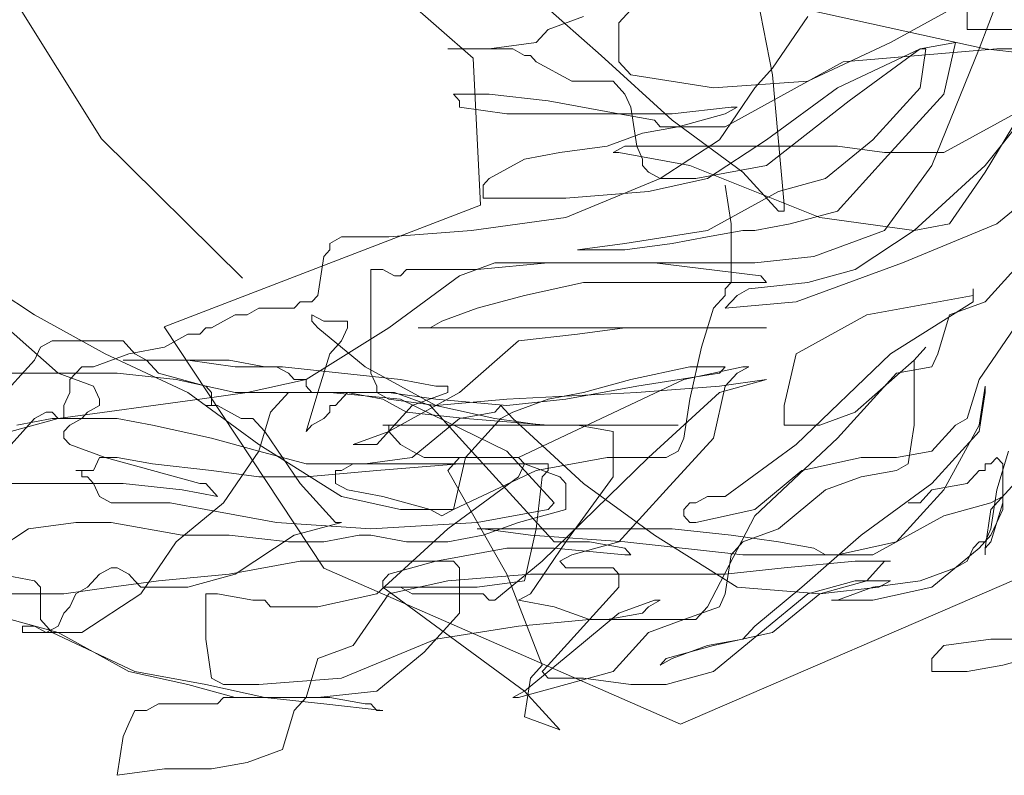
# Model space of a CAD drawing. Units: inches. Extents: x 1994 to 3075, y 3517 to 3950.
# Tile 38 of 58: x 1994.64257 to 1994.647842, y 3553.737841 to 3553.741889. Entities that reach past the tile are written whole.
import ezdxf

# ---------------------------------------------------------------- set-up
doc = ezdxf.new("R2010")
doc.units = ezdxf.units.IN
doc.layers.add('A-FURN-REFR', color=8, linetype='Continuous', lineweight=13)

msp = doc.modelspace()

# ---------------------------------------------------------------- linework, layer by layer
at = {"layer": 'A-FURN-REFR'}
for p, q in [((1994.6419152, 3553.7430024), (1994.6430076, 3553.7412502)), ((1994.6449987, 3553.7416831), (1994.6436467, 3553.7428672)), ((1994.6466007, 3553.741594), (1994.6464111, 3553.7425669)), ((1994.6480232, 3553.7425669), (1994.647707, 3553.741733)), ((1994.6476438, 3553.742289), (1994.6476438, 3553.7418372)), ((1994.6453679, 3553.7419762), (1994.645684, 3553.7416983)), ((1994.6476122, 3553.7419762), (1994.6472329, 3553.7417677)), ((1994.6453996, 3553.7418372), (1994.6455892, 3553.7419067)), ((1994.6457789, 3553.741872), (1994.6458421, 3553.7419415)), ((1994.6467904, 3553.7419067), (1994.6466007, 3553.7416288)), ((1994.6467904, 3553.7419415), (1994.6477386, 3553.741733)), ((1994.6453363, 3553.7417677), (1994.6453996, 3553.7418372)), ((1994.6457789, 3553.7416635), (1994.6457789, 3553.741872)), ((1994.6476438, 3553.7418372), (1994.6480548, 3553.7418372)), ((1994.6448622, 3553.741733), (1994.6450834, 3553.741733)), ((1994.6452099, 3553.741733), (1994.6448622, 3553.741733)), ((1994.6450834, 3553.741733), (1994.6453363, 3553.7417677)), ((1994.6452731, 3553.7416983), (1994.6452099, 3553.741733)), ((1994.6472329, 3553.7417677), (1994.6467904, 3553.7415593)), ((1994.6469484, 3553.7415245), (1994.647391, 3553.741733)), ((1994.6478019, 3553.741733), (1994.64698, 3553.7416635)), ((1994.647391, 3553.741733), (1994.6470116, 3553.741455)), ((1994.647391, 3553.741733), (1994.6475806, 3553.7417677)), ((1994.6474226, 3553.741733), (1994.647391, 3553.741733)), ((1994.647391, 3553.7415245), (1994.6474226, 3553.741733)), ((1994.647707, 3553.741733), (1994.6474542, 3553.7411075)), ((1994.6475806, 3553.7417677), (1994.6475174, 3553.7414898)), ((1994.6477386, 3553.741733), (1994.6483708, 3553.7416635)), ((1994.6483708, 3553.741733), (1994.6478019, 3553.741733)), ((1994.6450375, 3553.7408956), (1994.6449987, 3553.7416831)), ((1994.6453047, 3553.7416983), (1994.6452731, 3553.7416983)), ((1994.6453363, 3553.7416635), (1994.6453047, 3553.7416983)), ((1994.645684, 3553.7416983), (1994.6460633, 3553.7413508)), ((1994.645526, 3553.7415593), (1994.6453363, 3553.7416635)), ((1994.6458421, 3553.741594), (1994.6457789, 3553.7416635)), ((1994.64698, 3553.7416635), (1994.6463478, 3553.741316)), ((1994.6466007, 3553.7416288), (1994.6465059, 3553.7415245)), ((1994.6481812, 3553.7416635), (1994.6477386, 3553.7411075)), ((1994.6462846, 3553.7415245), (1994.6458421, 3553.741594)), ((1994.6466639, 3553.7408991), (1994.6466007, 3553.741594)), ((1994.6457472, 3553.7415593), (1994.645526, 3553.7415593)), ((1994.6458105, 3553.7414898), (1994.6457472, 3553.7415593)), ((1994.6467904, 3553.7415593), (1994.6462846, 3553.7415245)), ((1994.6465059, 3553.7415245), (1994.6463162, 3553.7412465)), ((1994.6465691, 3553.7412465), (1994.6469484, 3553.7415245)), ((1994.6471381, 3553.7412465), (1994.647391, 3553.7415245)), ((1994.6448938, 3553.7414898), (1994.6449254, 3553.741455)), ((1994.6450834, 3553.7414898), (1994.6448938, 3553.7414898)), ((1994.6453996, 3553.741455), (1994.6450834, 3553.7414898)), ((1994.6458421, 3553.7414202), (1994.6458105, 3553.7414898)), ((1994.6475174, 3553.7414898), (1994.6472013, 3553.7411423)), ((1994.6477386, 3553.7410728), (1994.6479915, 3553.7414898)), ((1994.6449254, 3553.741455), (1994.6449254, 3553.7414202)), ((1994.6449254, 3553.7414202), (1994.6451783, 3553.7413855)), ((1994.6457789, 3553.7413855), (1994.6453996, 3553.741455)), ((1994.6458737, 3553.7412118), (1994.6458421, 3553.7414202)), ((1994.6460633, 3553.7413855), (1994.6463794, 3553.7414202)), ((1994.6464111, 3553.7414202), (1994.6463478, 3553.7413855)), ((1994.6463794, 3553.7414202), (1994.6464111, 3553.7414202)), ((1994.6470116, 3553.741455), (1994.6465691, 3553.7411075)), ((1994.6480232, 3553.741455), (1994.6475174, 3553.741177)), ((1994.6451783, 3553.7413855), (1994.6460633, 3553.7413855)), ((1994.6459685, 3553.7413508), (1994.6457789, 3553.7413855)), ((1994.6463478, 3553.7413855), (1994.6460949, 3553.741316)), ((1994.6460949, 3553.741316), (1994.6459053, 3553.7412813)), ((1994.6460001, 3553.741316), (1994.6459685, 3553.7413508)), ((1994.6463478, 3553.741316), (1994.6460001, 3553.741316)), ((1994.6460633, 3553.7413508), (1994.6464427, 3553.7410728)), ((1994.6459053, 3553.7412813), (1994.6457156, 3553.7412118)), ((1994.6430076, 3553.7412502), (1994.643763, 3553.7405048)), ((1994.6457156, 3553.7412118), (1994.6454628, 3553.741177)), ((1994.6458105, 3553.7412118), (1994.6457472, 3553.741177)), ((1994.6469484, 3553.7412118), (1994.6458105, 3553.7412118)), ((1994.6459053, 3553.7411423), (1994.6458737, 3553.7412118)), ((1994.6463162, 3553.7412465), (1994.6460001, 3553.741038)), ((1994.646253, 3553.741038), (1994.6465691, 3553.7412465)), ((1994.6468852, 3553.741038), (1994.6471381, 3553.7412465)), ((1994.6472013, 3553.741177), (1994.6469484, 3553.7412118)), ((1994.6454628, 3553.741177), (1994.6452731, 3553.7411423)), ((1994.6457472, 3553.741177), (1994.6457789, 3553.741177)), ((1994.6457789, 3553.741177), (1994.6461582, 3553.7411075)), ((1994.6475174, 3553.741177), (1994.6472013, 3553.741177)), ((1994.6452731, 3553.7411423), (1994.6450834, 3553.741038)), ((1994.6459053, 3553.7411075), (1994.6459053, 3553.7411423)), ((1994.6459369, 3553.7410728), (1994.6459053, 3553.7411075)), ((1994.6461582, 3553.7411075), (1994.6468536, 3553.7408296)), ((1994.6465691, 3553.7411075), (1994.6461898, 3553.741038)), ((1994.6472013, 3553.7411423), (1994.6469484, 3553.7408643)), ((1994.6474542, 3553.7411075), (1994.6472013, 3553.7407601)), ((1994.6477386, 3553.7411075), (1994.6473593, 3553.7407601)), ((1994.6460001, 3553.741038), (1994.6459369, 3553.7410728)), ((1994.6464427, 3553.7410728), (1994.6466323, 3553.7408643)), ((1994.647549, 3553.7407948), (1994.6477386, 3553.7410728)), ((1994.6450834, 3553.741038), (1994.6450518, 3553.7410033)), ((1994.6450518, 3553.7410033), (1994.6450518, 3553.7409338)), ((1994.6460001, 3553.741038), (1994.6454944, 3553.7408296)), ((1994.6459369, 3553.7409686), (1994.646253, 3553.741038)), ((1994.6461898, 3553.741038), (1994.6460001, 3553.741038)), ((1994.6463794, 3553.7407948), (1994.6463478, 3553.7410033)), ((1994.6466323, 3553.7409686), (1994.6468852, 3553.741038)), ((1994.6478019, 3553.7407948), (1994.6480548, 3553.7410033)), ((1994.6454944, 3553.7409338), (1994.6459369, 3553.7409686)), ((1994.646253, 3553.7407601), (1994.6466323, 3553.7409686)), ((1994.6433447, 3553.7402433), (1994.6450375, 3553.7408956)), ((1994.6450518, 3553.7409338), (1994.6454944, 3553.7409338)), ((1994.6466639, 3553.7408643), (1994.6466639, 3553.7408991)), ((1994.6466323, 3553.7408643), (1994.6466639, 3553.7408643)), ((1994.6469484, 3553.7408643), (1994.6466955, 3553.7407948)), ((1994.6454944, 3553.7408296), (1994.6449886, 3553.7407601)), ((1994.6463794, 3553.7404821), (1994.6463794, 3553.7407948)), ((1994.6466955, 3553.7407948), (1994.6465059, 3553.7407601)), ((1994.6468536, 3553.7408296), (1994.6473593, 3553.7407601)), ((1994.6472961, 3553.7405864), (1994.6478019, 3553.7407948)), ((1994.6473593, 3553.7407601), (1994.647549, 3553.7407948)), ((1994.6449886, 3553.7407601), (1994.6445461, 3553.7407253)), ((1994.6458105, 3553.7406905), (1994.646253, 3553.7407601)), ((1994.6464427, 3553.7407601), (1994.646253, 3553.7407253)), ((1994.6465059, 3553.7407601), (1994.6464427, 3553.7407601)), ((1994.6472013, 3553.7407601), (1994.6470116, 3553.7406905)), ((1994.6473593, 3553.7407601), (1994.6470433, 3553.7405516)), ((1994.6442932, 3553.7407253), (1994.64423, 3553.7406905)), ((1994.64423, 3553.7406905), (1994.64423, 3553.7406558)), ((1994.6445461, 3553.7407253), (1994.6442932, 3553.7407253)), ((1994.6455576, 3553.7406558), (1994.6458105, 3553.7406905)), ((1994.6460633, 3553.7406905), (1994.6458105, 3553.7406558)), ((1994.646253, 3553.7407253), (1994.6460633, 3553.7406905)), ((1994.6470116, 3553.7406905), (1994.646822, 3553.7406211)), ((1994.64423, 3553.7406558), (1994.6441984, 3553.7406211)), ((1994.6458105, 3553.7406558), (1994.6455576, 3553.7406558)), ((1994.6441984, 3553.7406211), (1994.6441668, 3553.7404126)), ((1994.645115, 3553.7405864), (1994.6449254, 3553.7405168)), ((1994.6453996, 3553.7405864), (1994.6450202, 3553.7405516)), ((1994.6465059, 3553.7405864), (1994.645115, 3553.7405864)), ((1994.6459685, 3553.7405864), (1994.6453996, 3553.7405864)), ((1994.6465375, 3553.7405168), (1994.6459685, 3553.7405864)), ((1994.646822, 3553.7406211), (1994.6465059, 3553.7405864)), ((1994.6467271, 3553.7403778), (1994.6472961, 3553.7405864)), ((1994.6477386, 3553.7403778), (1994.6479283, 3553.7405864)), ((1994.6444512, 3553.7405516), (1994.6444512, 3553.7399956)), ((1994.6445145, 3553.7405516), (1994.6444512, 3553.7405516)), ((1994.6445777, 3553.7405168), (1994.6445145, 3553.7405516)), ((1994.6446409, 3553.7405516), (1994.6446093, 3553.7405168)), ((1994.6450202, 3553.7405516), (1994.6446409, 3553.7405516)), ((1994.6470433, 3553.7405516), (1994.6467904, 3553.7404821)), ((1994.6423334, 3553.7405168), (1994.6426495, 3553.7403083)), ((1994.6449254, 3553.7405168), (1994.6445461, 3553.7402389)), ((1994.6446093, 3553.7405168), (1994.6445777, 3553.7405168)), ((1994.6452731, 3553.7404126), (1994.6455892, 3553.7404821)), ((1994.6455892, 3553.7404821), (1994.6465691, 3553.7404821)), ((1994.6463478, 3553.7404473), (1994.6463794, 3553.7404821)), ((1994.6467904, 3553.7404821), (1994.6464743, 3553.7404473)), ((1994.6465691, 3553.7404821), (1994.6465375, 3553.7405168)), ((1994.6463478, 3553.7404126), (1994.6463478, 3553.7404473)), ((1994.6464743, 3553.7404473), (1994.6464111, 3553.7404126)), ((1994.6476754, 3553.7404473), (1994.6476754, 3553.7403778)), ((1994.6476754, 3553.7404126), (1994.6476754, 3553.7404473)), ((1994.6440719, 3553.7403778), (1994.6440403, 3553.7403431)), ((1994.6441351, 3553.7403778), (1994.6440719, 3553.7403778)), ((1994.6441668, 3553.7404126), (1994.6441351, 3553.7403778)), ((1994.6450202, 3553.7403431), (1994.6452731, 3553.7404126)), ((1994.6462846, 3553.7403431), (1994.6463478, 3553.7404126)), ((1994.6464111, 3553.7404126), (1994.6463478, 3553.7403431)), ((1994.6463478, 3553.7403431), (1994.6467271, 3553.7403778)), ((1994.6471065, 3553.7403083), (1994.6476754, 3553.7404126)), ((1994.6476754, 3553.7403778), (1994.6472329, 3553.7400999)), ((1994.647549, 3553.7403083), (1994.6477386, 3553.7403778)), ((1994.6426495, 3553.7403083), (1994.6430288, 3553.7400999)), ((1994.6437242, 3553.7403083), (1994.643661, 3553.7402736)), ((1994.6437875, 3553.7403083), (1994.6437242, 3553.7403083)), ((1994.6438507, 3553.7403431), (1994.6437875, 3553.7403083)), ((1994.6440403, 3553.7403431), (1994.6438507, 3553.7403431)), ((1994.6441351, 3553.7403083), (1994.6441351, 3553.7402736)), ((1994.6441984, 3553.7402736), (1994.6441351, 3553.7403083)), ((1994.6448306, 3553.7402736), (1994.6450202, 3553.7403431)), ((1994.6462214, 3553.7401346), (1994.6462846, 3553.7403431)), ((1994.6467271, 3553.7400999), (1994.6471065, 3553.7403083)), ((1994.6474858, 3553.7400999), (1994.647549, 3553.7403083)), ((1994.642776, 3553.7399956), (1994.6424598, 3553.7402736)), ((1994.643661, 3553.7402736), (1994.6435978, 3553.7402389)), ((1994.6441351, 3553.7402736), (1994.6441668, 3553.7402389)), ((1994.6443248, 3553.7402736), (1994.6441984, 3553.7402736)), ((1994.6443248, 3553.7402389), (1994.6443248, 3553.7402736)), ((1994.6447673, 3553.7402389), (1994.6448306, 3553.7402736)), ((1994.6441989, 3553.7389509), (1994.6433447, 3553.7402433)), ((1994.6434713, 3553.7402041), (1994.6433449, 3553.7401346)), ((1994.6435346, 3553.7402041), (1994.6434713, 3553.7402041)), ((1994.6435662, 3553.7402389), (1994.6435346, 3553.7402041)), ((1994.6435978, 3553.7402389), (1994.6435662, 3553.7402389)), ((1994.6445461, 3553.7402389), (1994.6441035, 3553.7399609)), ((1994.6441668, 3553.7402389), (1994.6444196, 3553.7400304)), ((1994.6442932, 3553.7401694), (1994.6443248, 3553.7402389)), ((1994.6447041, 3553.7402389), (1994.6447673, 3553.7402389)), ((1994.6465691, 3553.7402389), (1994.6447041, 3553.7402389)), ((1994.6452415, 3553.7401694), (1994.6455576, 3553.7402041)), ((1994.6455576, 3553.7402041), (1994.6458105, 3553.7402389)), ((1994.6458105, 3553.7402389), (1994.6465691, 3553.7402389)), ((1994.647707, 3553.7399609), (1994.6478967, 3553.7402389)), ((1994.6426811, 3553.7401346), (1994.6427443, 3553.7401694)), ((1994.6427443, 3553.7401694), (1994.6431236, 3553.7401694)), ((1994.6431236, 3553.7401694), (1994.6431869, 3553.7400999)), ((1994.64423, 3553.7400999), (1994.6442932, 3553.7401694)), ((1994.6449254, 3553.7398914), (1994.6452415, 3553.7401694)), ((1994.6426495, 3553.7400651), (1994.6426811, 3553.7401346)), ((1994.6431553, 3553.7400999), (1994.6429656, 3553.7400304)), ((1994.6430288, 3553.7400999), (1994.6434713, 3553.7398914)), ((1994.6433449, 3553.7401346), (1994.6431553, 3553.7400999)), ((1994.6431869, 3553.7400999), (1994.6432501, 3553.7400651)), ((1994.6441668, 3553.7398914), (1994.64423, 3553.7400999)), ((1994.6461582, 3553.7398567), (1994.6462214, 3553.7401346)), ((1994.6466639, 3553.7398219), (1994.6467271, 3553.7400999)), ((1994.6472329, 3553.7400999), (1994.6467271, 3553.7396134)), ((1994.6474226, 3553.7401346), (1994.6473593, 3553.7400651)), ((1994.6473593, 3553.7400651), (1994.6474226, 3553.7401346)), ((1994.6474542, 3553.7400304), (1994.6474858, 3553.7400999)), ((1994.6423966, 3553.7397872), (1994.6426495, 3553.7400651)), ((1994.6431236, 3553.7400651), (1994.6434713, 3553.7400651)), ((1994.6436926, 3553.7400651), (1994.6431236, 3553.7400651)), ((1994.6432501, 3553.7400651), (1994.6433133, 3553.7399956)), ((1994.6434713, 3553.7400651), (1994.6437242, 3553.7400304)), ((1994.6438823, 3553.7400304), (1994.6436926, 3553.7400651)), ((1994.6473593, 3553.7400651), (1994.6470433, 3553.7397872)), ((1994.6473593, 3553.7397176), (1994.6473593, 3553.7400651)), ((1994.6420173, 3553.7399956), (1994.643092, 3553.7399956)), ((1994.6429656, 3553.7399262), (1994.642776, 3553.7399956)), ((1994.6429024, 3553.7400304), (1994.6428392, 3553.7399609)), ((1994.6429656, 3553.7400304), (1994.6429024, 3553.7400304)), ((1994.643092, 3553.7399956), (1994.6434081, 3553.7399609)), ((1994.6433133, 3553.7399956), (1994.6435662, 3553.7399262)), ((1994.6437242, 3553.7400304), (1994.6439771, 3553.7400304)), ((1994.6439455, 3553.7400304), (1994.6438823, 3553.7400304)), ((1994.6440087, 3553.7399956), (1994.6439455, 3553.7400304)), ((1994.6439771, 3553.7400304), (1994.6442932, 3553.7399956)), ((1994.6440403, 3553.7399609), (1994.6440087, 3553.7399956)), ((1994.6442932, 3553.7399956), (1994.6446093, 3553.7399609)), ((1994.6444196, 3553.7400304), (1994.644799, 3553.7398219)), ((1994.6444512, 3553.7399956), (1994.6444829, 3553.7399262)), ((1994.6458421, 3553.7399609), (1994.6461582, 3553.7400304)), ((1994.6463162, 3553.7399956), (1994.6458737, 3553.7399262)), ((1994.6464427, 3553.7400304), (1994.6461265, 3553.7399609)), ((1994.6461582, 3553.7400304), (1994.6463478, 3553.7400304)), ((1994.6463478, 3553.7400304), (1994.6463162, 3553.7399956)), ((1994.6463478, 3553.7399262), (1994.6464111, 3553.7399956)), ((1994.6464111, 3553.7399956), (1994.6464743, 3553.7400304)), ((1994.6464743, 3553.7400304), (1994.6464427, 3553.7400304)), ((1994.6469484, 3553.7396481), (1994.6472645, 3553.7399956)), ((1994.6472645, 3553.7399956), (1994.6474542, 3553.7400304)), ((1994.6428392, 3553.7399609), (1994.6428392, 3553.7398914)), ((1994.6434081, 3553.7399609), (1994.6437242, 3553.7398914)), ((1994.6441035, 3553.7399609), (1994.6437875, 3553.7398914)), ((1994.6441035, 3553.7399609), (1994.6440403, 3553.7399609)), ((1994.6441035, 3553.7399262), (1994.6441035, 3553.7399609)), ((1994.6446093, 3553.7399609), (1994.644799, 3553.7399262)), ((1994.6455892, 3553.7398914), (1994.6458421, 3553.7399609)), ((1994.6461265, 3553.7399609), (1994.645684, 3553.7397524)), ((1994.6465691, 3553.7399609), (1994.6463162, 3553.7398914)), ((1994.6463162, 3553.7399262), (1994.6465691, 3553.7399609)), ((1994.6476438, 3553.7397524), (1994.647707, 3553.7399609)), ((1994.6428392, 3553.7398914), (1994.6428076, 3553.7398219)), ((1994.6429972, 3553.7398567), (1994.6429656, 3553.7399262)), ((1994.6434713, 3553.7398914), (1994.6438507, 3553.7396134)), ((1994.6437875, 3553.7398914), (1994.6435346, 3553.7398567)), ((1994.6435662, 3553.7399262), (1994.6435978, 3553.7398914)), ((1994.6435978, 3553.7398914), (1994.6435978, 3553.7398219)), ((1994.6437242, 3553.7398914), (1994.64423, 3553.7398914)), ((1994.6439139, 3553.7397872), (1994.6440087, 3553.7398914)), ((1994.6440087, 3553.7398914), (1994.6445777, 3553.7398914)), ((1994.6441351, 3553.7398914), (1994.6441035, 3553.7399262)), ((1994.6441035, 3553.7396829), (1994.6441668, 3553.7398914)), ((1994.6443248, 3553.7398914), (1994.6441351, 3553.7398914)), ((1994.64423, 3553.7398914), (1994.6446093, 3553.7398567)), ((1994.6443248, 3553.7398914), (1994.6442616, 3553.7398219)), ((1994.6445461, 3553.7398914), (1994.6443248, 3553.7398914)), ((1994.6445145, 3553.7398567), (1994.6443248, 3553.7398914)), ((1994.6444829, 3553.7399262), (1994.6444829, 3553.7398914)), ((1994.6444829, 3553.7398914), (1994.6445461, 3553.7398567)), ((1994.644799, 3553.7398567), (1994.6445461, 3553.7398914)), ((1994.6445461, 3553.7396829), (1994.6449254, 3553.7398914)), ((1994.6445777, 3553.7398914), (1994.6447673, 3553.7398219)), ((1994.6448622, 3553.7398914), (1994.6446725, 3553.7398219)), ((1994.644799, 3553.7399262), (1994.6448622, 3553.7399262)), ((1994.6448622, 3553.7399262), (1994.6448622, 3553.7398914)), ((1994.6451783, 3553.7398567), (1994.6458737, 3553.7398914)), ((1994.6453996, 3553.7398567), (1994.6455892, 3553.7398914)), ((1994.6458737, 3553.7399262), (1994.6454944, 3553.7398567)), ((1994.6458737, 3553.7398914), (1994.6463162, 3553.7399262)), ((1994.6463162, 3553.7398914), (1994.6459369, 3553.7395439)), ((1994.6462846, 3553.7396481), (1994.6463478, 3553.7399262)), ((1994.647707, 3553.7397176), (1994.6477386, 3553.7399262)), ((1994.6477386, 3553.7398914), (1994.647707, 3553.7396829)), ((1994.6477386, 3553.7399262), (1994.6477386, 3553.7398914)), ((1994.6435346, 3553.7398567), (1994.642776, 3553.7397524)), ((1994.6429972, 3553.7398219), (1994.6429972, 3553.7398567)), ((1994.6446409, 3553.7397872), (1994.6445145, 3553.7398567)), ((1994.6445461, 3553.7398567), (1994.644799, 3553.7398219)), ((1994.6446093, 3553.7398567), (1994.6451783, 3553.7395786)), ((1994.6451783, 3553.7398219), (1994.644799, 3553.7398567)), ((1994.644799, 3553.7398219), (1994.6451783, 3553.7398567)), ((1994.6454944, 3553.7398567), (1994.6451783, 3553.7398219)), ((1994.6452099, 3553.7397872), (1994.6453996, 3553.7398567)), ((1994.6461265, 3553.7396481), (1994.6461582, 3553.7398567)), ((1994.6427127, 3553.7397872), (1994.6426495, 3553.7397524)), ((1994.6427443, 3553.7397872), (1994.6427127, 3553.7397872)), ((1994.642776, 3553.7397524), (1994.6427443, 3553.7397872)), ((1994.6428076, 3553.7398219), (1994.6428076, 3553.7397524)), ((1994.6429024, 3553.7397524), (1994.642934, 3553.7397872)), ((1994.642934, 3553.7397872), (1994.6429972, 3553.7398219)), ((1994.6435662, 3553.7398219), (1994.6436294, 3553.7398219)), ((1994.6435978, 3553.7398219), (1994.6435662, 3553.7398219)), ((1994.6436294, 3553.7398219), (1994.6437558, 3553.7397524)), ((1994.6438507, 3553.7395786), (1994.6439139, 3553.7397872)), ((1994.64423, 3553.7397872), (1994.6441984, 3553.7397524)), ((1994.64423, 3553.7398219), (1994.64423, 3553.7397872)), ((1994.6442616, 3553.7398219), (1994.64423, 3553.7398219)), ((1994.6446725, 3553.7398219), (1994.6444829, 3553.7396134)), ((1994.644957, 3553.7397524), (1994.6446409, 3553.7397872)), ((1994.6447673, 3553.7398219), (1994.644957, 3553.7396134)), ((1994.644799, 3553.7398219), (1994.645115, 3553.7397524)), ((1994.645115, 3553.7397872), (1994.6449254, 3553.7397524)), ((1994.6451466, 3553.7398219), (1994.645115, 3553.7397872)), ((1994.6452099, 3553.7397524), (1994.6451466, 3553.7398219)), ((1994.6451466, 3553.7397524), (1994.6452099, 3553.7397872)), ((1994.6466639, 3553.7397176), (1994.6466639, 3553.7398219)), ((1994.6470433, 3553.7397872), (1994.6468536, 3553.7397176)), ((1994.6426495, 3553.7397524), (1994.6424598, 3553.7395439)), ((1994.642776, 3553.7397524), (1994.642523, 3553.7396829)), ((1994.6427443, 3553.7397524), (1994.6425547, 3553.7397176)), ((1994.643092, 3553.7397524), (1994.6427443, 3553.7397524)), ((1994.6428076, 3553.7397524), (1994.642776, 3553.7397524)), ((1994.6428392, 3553.7397176), (1994.6429024, 3553.7397524)), ((1994.6432817, 3553.7397176), (1994.643092, 3553.7397524)), ((1994.6437558, 3553.7397524), (1994.6438191, 3553.7397524)), ((1994.6438191, 3553.7397524), (1994.6438823, 3553.7396829)), ((1994.6441984, 3553.7397524), (1994.6441351, 3553.7397176)), ((1994.6449254, 3553.7397524), (1994.6446725, 3553.7395439)), ((1994.644957, 3553.7395439), (1994.6451466, 3553.7397524)), ((1994.6453996, 3553.7397176), (1994.644957, 3553.7397524)), ((1994.645115, 3553.7397524), (1994.6453679, 3553.7397176)), ((1994.6455892, 3553.7394049), (1994.6452099, 3553.7397524)), ((1994.645684, 3553.7397524), (1994.6452415, 3553.7395439)), ((1994.6475806, 3553.7397176), (1994.6476438, 3553.7397524)), ((1994.6428076, 3553.7396829), (1994.6428392, 3553.7397176)), ((1994.6428076, 3553.7396481), (1994.6428076, 3553.7396829)), ((1994.6435978, 3553.7396481), (1994.6432817, 3553.7397176)), ((1994.6438823, 3553.7396829), (1994.6440719, 3553.7394049)), ((1994.6441351, 3553.7397176), (1994.6441035, 3553.7396829)), ((1994.6443564, 3553.7396134), (1994.6445461, 3553.7396829)), ((1994.6445145, 3553.7397176), (1994.6460949, 3553.7397176)), ((1994.6445461, 3553.7397176), (1994.6445145, 3553.7397176)), ((1994.6445461, 3553.7396829), (1994.6445461, 3553.7397176)), ((1994.6446093, 3553.7396134), (1994.6445461, 3553.7396829)), ((1994.6453679, 3553.7397176), (1994.6455576, 3553.7397176)), ((1994.6460949, 3553.7397176), (1994.6453996, 3553.7397176)), ((1994.6455576, 3553.7397176), (1994.6457472, 3553.7396829)), ((1994.6457472, 3553.7396829), (1994.6457472, 3553.7394397)), ((1994.6468536, 3553.7397176), (1994.6466639, 3553.7397176)), ((1994.6473277, 3553.7395092), (1994.6473593, 3553.7397176)), ((1994.6474542, 3553.7395786), (1994.6475806, 3553.7397176)), ((1994.647707, 3553.7396829), (1994.6474542, 3553.7394049)), ((1994.6475174, 3553.7393702), (1994.647707, 3553.7397176)), ((1994.6428392, 3553.7396134), (1994.6428076, 3553.7396481)), ((1994.6438507, 3553.7395786), (1994.6435978, 3553.7396481)), ((1994.6460317, 3553.7393702), (1994.6462846, 3553.7396481)), ((1994.6460949, 3553.7395786), (1994.6461265, 3553.7396481)), ((1994.6465059, 3553.7392312), (1994.6469484, 3553.7396481)), ((1994.6430288, 3553.7395439), (1994.6428392, 3553.7396134)), ((1994.643661, 3553.7393007), (1994.6438507, 3553.7395786)), ((1994.6438507, 3553.7396134), (1994.6442932, 3553.7393354)), ((1994.6441035, 3553.7395092), (1994.6438507, 3553.7395786)), ((1994.6444829, 3553.7396134), (1994.6443564, 3553.7396134)), ((1994.6446725, 3553.7395786), (1994.6446093, 3553.7396134)), ((1994.6447357, 3553.7395439), (1994.6446725, 3553.7395786)), ((1994.644957, 3553.7396134), (1994.6452099, 3553.7393354)), ((1994.6451783, 3553.7395786), (1994.6454312, 3553.7393007)), ((1994.6460317, 3553.7395439), (1994.6460949, 3553.7395786)), ((1994.6467271, 3553.7396134), (1994.6463478, 3553.7393354)), ((1994.6472645, 3553.7395439), (1994.6474542, 3553.7395786)), ((1994.6478651, 3553.7395786), (1994.6478019, 3553.7393702)), ((1994.6429656, 3553.7394744), (1994.6429972, 3553.7395439)), ((1994.6429972, 3553.7395439), (1994.643092, 3553.7395439)), ((1994.6435346, 3553.7394049), (1994.6430288, 3553.7395439)), ((1994.643092, 3553.7395439), (1994.6432817, 3553.7395092)), ((1994.6446725, 3553.7395439), (1994.6444196, 3553.7395092)), ((1994.6452415, 3553.7395439), (1994.6447357, 3553.7395439)), ((1994.6448622, 3553.7394744), (1994.6449254, 3553.7395439)), ((1994.6448938, 3553.7392659), (1994.644957, 3553.7395439)), ((1994.6449254, 3553.7395439), (1994.6452415, 3553.7395439)), ((1994.6452415, 3553.7395439), (1994.6452731, 3553.7395092)), ((1994.6453363, 3553.7394744), (1994.6457156, 3553.7395439)), ((1994.6459369, 3553.7395439), (1994.6453679, 3553.738988)), ((1994.6457156, 3553.7395439), (1994.6460317, 3553.7395439)), ((1994.6467587, 3553.7394744), (1994.6470749, 3553.7395439)), ((1994.6470749, 3553.7395439), (1994.6472645, 3553.7395439)), ((1994.6477703, 3553.7395092), (1994.6478019, 3553.7395439)), ((1994.6478019, 3553.7395439), (1994.6478335, 3553.7395092)), ((1994.6428708, 3553.7394744), (1994.6429656, 3553.7394744)), ((1994.6429024, 3553.7394744), (1994.6428708, 3553.7394744)), ((1994.6429024, 3553.7394397), (1994.6429024, 3553.7394744)), ((1994.6432817, 3553.7395092), (1994.6435978, 3553.7394744)), ((1994.6435978, 3553.7394744), (1994.6438507, 3553.7394397)), ((1994.6444196, 3553.7395092), (1994.6441035, 3553.7395092)), ((1994.6441035, 3553.7394397), (1994.6444829, 3553.7394744)), ((1994.6442616, 3553.7394744), (1994.6442616, 3553.7394049)), ((1994.6442932, 3553.7394744), (1994.6442616, 3553.7394744)), ((1994.6443564, 3553.7395092), (1994.6442932, 3553.7394744)), ((1994.6453996, 3553.7395092), (1994.6443564, 3553.7395092)), ((1994.6444829, 3553.7394744), (1994.6449254, 3553.7395092)), ((1994.6451783, 3553.7389184), (1994.6448622, 3553.7394744)), ((1994.6448938, 3553.7392659), (1994.6453363, 3553.7394744)), ((1994.6449254, 3553.7395092), (1994.6452731, 3553.7395092)), ((1994.6452731, 3553.7395092), (1994.6452415, 3553.7394397)), ((1994.6452731, 3553.7395092), (1994.6454628, 3553.7394397)), ((1994.6453679, 3553.7394397), (1994.6453996, 3553.7394744)), ((1994.6453996, 3553.7394744), (1994.6453996, 3553.7395092)), ((1994.6465059, 3553.7392659), (1994.6467587, 3553.7394744)), ((1994.6470749, 3553.7394397), (1994.6472645, 3553.7394744)), ((1994.6472645, 3553.7394744), (1994.6473277, 3553.7395092)), ((1994.6476438, 3553.7394049), (1994.647707, 3553.7394744)), ((1994.647707, 3553.7394744), (1994.6477386, 3553.7394744)), ((1994.6477386, 3553.7395092), (1994.6477703, 3553.7395092)), ((1994.6477386, 3553.7394744), (1994.6477386, 3553.7395092)), ((1994.6477703, 3553.7392659), (1994.6479599, 3553.7394744)), ((1994.6478335, 3553.7395092), (1994.6478335, 3553.7393007)), ((1994.642934, 3553.7394397), (1994.6429024, 3553.7394397)), ((1994.6429656, 3553.7394049), (1994.642934, 3553.7394397)), ((1994.6438507, 3553.7394397), (1994.6441035, 3553.7394397)), ((1994.6452415, 3553.7394397), (1994.6448622, 3553.7391617)), ((1994.6453363, 3553.7391617), (1994.6453679, 3553.7394397)), ((1994.6454628, 3553.7394397), (1994.6454944, 3553.7394049)), ((1994.6457472, 3553.7394397), (1994.6454944, 3553.7390922)), ((1994.6468852, 3553.7393702), (1994.6470749, 3553.7394397)), ((1994.6419857, 3553.7394049), (1994.6431236, 3553.7394049)), ((1994.6429972, 3553.7393354), (1994.6429656, 3553.7394049)), ((1994.6431236, 3553.7394049), (1994.6434397, 3553.7393702)), ((1994.6434397, 3553.7393702), (1994.6436294, 3553.7393354)), ((1994.6435662, 3553.7394049), (1994.6435346, 3553.7394049)), ((1994.6436294, 3553.7393354), (1994.6435662, 3553.7394049)), ((1994.6440719, 3553.7394049), (1994.6442616, 3553.7391965)), ((1994.6442616, 3553.7394049), (1994.6443248, 3553.7393702)), ((1994.6443248, 3553.7393702), (1994.6445145, 3553.7393354)), ((1994.6454944, 3553.7394049), (1994.6454944, 3553.7392659)), ((1994.6459685, 3553.739127), (1994.6455892, 3553.7394049)), ((1994.6457789, 3553.7390922), (1994.6460317, 3553.7393702)), ((1994.6466323, 3553.7391617), (1994.6468852, 3553.7393702)), ((1994.6474542, 3553.7394049), (1994.6470749, 3553.739127)), ((1994.6472645, 3553.7390922), (1994.6475174, 3553.7393702)), ((1994.647391, 3553.7393007), (1994.6474542, 3553.7393702)), ((1994.6474542, 3553.7393702), (1994.6476438, 3553.7394049)), ((1994.6478019, 3553.7393702), (1994.6477703, 3553.7391617)), ((1994.6430604, 3553.7393007), (1994.6429972, 3553.7393354)), ((1994.6442932, 3553.7393354), (1994.6446093, 3553.7392659)), ((1994.6445145, 3553.7393354), (1994.6447673, 3553.7392659)), ((1994.6452099, 3553.7393354), (1994.6453996, 3553.739127)), ((1994.646253, 3553.7393354), (1994.6461898, 3553.7393007)), ((1994.6463478, 3553.7393354), (1994.646253, 3553.7393354)), ((1994.6478335, 3553.7393354), (1994.6477703, 3553.7393007)), ((1994.6478335, 3553.7392659), (1994.6478335, 3553.7393354)), ((1994.6433765, 3553.7393007), (1994.6430604, 3553.7393007)), ((1994.6435662, 3553.7392659), (1994.6433765, 3553.7393007)), ((1994.6434081, 3553.7390922), (1994.643661, 3553.7393007)), ((1994.6439455, 3553.7391965), (1994.6435662, 3553.7392659)), ((1994.6446093, 3553.7392659), (1994.6448938, 3553.7392659)), ((1994.6447673, 3553.7392659), (1994.6448306, 3553.7392312)), ((1994.6448306, 3553.7392312), (1994.6448938, 3553.7392659)), ((1994.6453996, 3553.7392659), (1994.6450202, 3553.7391965)), ((1994.6454944, 3553.7392659), (1994.6452415, 3553.7391965)), ((1994.6454312, 3553.7393007), (1994.6453996, 3553.7392659)), ((1994.6461582, 3553.7393007), (1994.6461265, 3553.7392659)), ((1994.6461265, 3553.7392659), (1994.6461265, 3553.7392312)), ((1994.6461898, 3553.7393007), (1994.6461582, 3553.7393007)), ((1994.6461898, 3553.7391965), (1994.6465059, 3553.7392659)), ((1994.6473277, 3553.7393007), (1994.647391, 3553.7393007)), ((1994.6477703, 3553.7393007), (1994.6475174, 3553.7392312)), ((1994.6477386, 3553.7390575), (1994.6477703, 3553.7392659)), ((1994.6478335, 3553.7393007), (1994.6477703, 3553.7390922)), ((1994.6478019, 3553.7391965), (1994.6478335, 3553.7392659)), ((1994.6461265, 3553.7392312), (1994.6461582, 3553.7391965)), ((1994.646253, 3553.7387447), (1994.6465059, 3553.7392312)), ((1994.6475174, 3553.7392312), (1994.6471381, 3553.7390227)), ((1994.6426179, 3553.7391617), (1994.6423018, 3553.7389532)), ((1994.6428708, 3553.7391965), (1994.6426179, 3553.7391617)), ((1994.6430604, 3553.7391965), (1994.6428708, 3553.7391965)), ((1994.6434397, 3553.739127), (1994.6430604, 3553.7391965)), ((1994.6444512, 3553.7391617), (1994.6439455, 3553.7391965)), ((1994.6442932, 3553.7391965), (1994.6440403, 3553.739127)), ((1994.6442616, 3553.7391965), (1994.6442932, 3553.7391965)), ((1994.6450202, 3553.7391965), (1994.6444512, 3553.7391617)), ((1994.6448622, 3553.7391617), (1994.6444829, 3553.7388143)), ((1994.6450202, 3553.7391617), (1994.6450518, 3553.7391617)), ((1994.6460633, 3553.7391617), (1994.6450202, 3553.7391617)), ((1994.6452415, 3553.7391965), (1994.6450518, 3553.739127)), ((1994.6450518, 3553.7391617), (1994.6453047, 3553.739127)), ((1994.6452731, 3553.7388837), (1994.6453363, 3553.7391617)), ((1994.6463794, 3553.739127), (1994.6460633, 3553.7391617)), ((1994.6461582, 3553.7391965), (1994.6461898, 3553.7391965)), ((1994.6464427, 3553.7390922), (1994.6466323, 3553.7391617)), ((1994.6477703, 3553.7391617), (1994.6477386, 3553.7390922)), ((1994.6477703, 3553.739127), (1994.6478019, 3553.7391965)), ((1994.6436926, 3553.739127), (1994.6434397, 3553.739127)), ((1994.6440087, 3553.7390922), (1994.6436926, 3553.739127)), ((1994.6440403, 3553.739127), (1994.6437242, 3553.7389184)), ((1994.644388, 3553.739127), (1994.6441984, 3553.7390922)), ((1994.6444512, 3553.739127), (1994.644388, 3553.739127)), ((1994.6446409, 3553.7390922), (1994.6444512, 3553.739127)), ((1994.6450518, 3553.739127), (1994.6448622, 3553.7390922)), ((1994.6453047, 3553.739127), (1994.6458105, 3553.7390922)), ((1994.6453996, 3553.739127), (1994.6454312, 3553.7390922)), ((1994.6464111, 3553.738849), (1994.6459685, 3553.739127)), ((1994.6466323, 3553.7390922), (1994.6463794, 3553.739127)), ((1994.6470749, 3553.739127), (1994.6467587, 3553.738849)), ((1994.647707, 3553.7390575), (1994.6477703, 3553.739127)), ((1994.6432185, 3553.7388143), (1994.6434081, 3553.7390922)), ((1994.6441984, 3553.7390922), (1994.6440087, 3553.7390922)), ((1994.6448622, 3553.7390922), (1994.6446409, 3553.7390922)), ((1994.6451783, 3553.7390575), (1994.644799, 3553.738988)), ((1994.6454312, 3553.7390575), (1994.6451783, 3553.7390575)), ((1994.6454944, 3553.7390922), (1994.6453047, 3553.7388143)), ((1994.6454312, 3553.7390922), (1994.6456208, 3553.7390922)), ((1994.6458105, 3553.7390227), (1994.6454312, 3553.7390575)), ((1994.645526, 3553.7390227), (1994.6457789, 3553.7390922)), ((1994.6456208, 3553.7390922), (1994.6458105, 3553.7390575)), ((1994.6458105, 3553.7390922), (1994.6464427, 3553.7390227)), ((1994.6458105, 3553.7390575), (1994.6458421, 3553.7390227)), ((1994.6463794, 3553.7390227), (1994.6464427, 3553.7390922)), ((1994.646822, 3553.7390575), (1994.6466323, 3553.7390922)), ((1994.6468852, 3553.7390227), (1994.646822, 3553.7390575)), ((1994.6469484, 3553.7390227), (1994.6472645, 3553.7390922)), ((1994.6474542, 3553.738849), (1994.647707, 3553.7390575)), ((1994.6476754, 3553.7390575), (1994.6476438, 3553.738988)), ((1994.647707, 3553.7390922), (1994.6476754, 3553.7390575)), ((1994.6477386, 3553.7390922), (1994.647707, 3553.7390922)), ((1994.6477703, 3553.7390922), (1994.6477386, 3553.7390575)), ((1994.6477386, 3553.7390227), (1994.6477386, 3553.7390575)), ((1994.6477386, 3553.7390575), (1994.6477386, 3553.7390227)), ((1994.6454628, 3553.738988), (1994.645526, 3553.7390227)), ((1994.6458421, 3553.7390227), (1994.6458105, 3553.7390227)), ((1994.6482198, 3553.7390294), (1994.6461087, 3553.7381155)), ((1994.6463478, 3553.7388143), (1994.6463794, 3553.7390227)), ((1994.6464427, 3553.7390227), (1994.6469484, 3553.7390227)), ((1994.6471381, 3553.7390227), (1994.6468852, 3553.7390227)), ((1994.6430604, 3553.7389532), (1994.6429972, 3553.7389184)), ((1994.643092, 3553.7389532), (1994.6430604, 3553.7389532)), ((1994.6431553, 3553.7389184), (1994.643092, 3553.7389532)), ((1994.6436926, 3553.7389184), (1994.6440719, 3553.738988)), ((1994.6440719, 3553.738988), (1994.6448938, 3553.738988)), ((1994.6461087, 3553.7381155), (1994.6441989, 3553.7389509)), ((1994.644799, 3553.738988), (1994.6445461, 3553.7389184)), ((1994.6448938, 3553.738988), (1994.6449254, 3553.7389532)), ((1994.6449254, 3553.7389532), (1994.6449254, 3553.73871)), ((1994.6453679, 3553.738988), (1994.645115, 3553.7387795)), ((1994.6454944, 3553.7389532), (1994.6454628, 3553.738988)), ((1994.6457472, 3553.7389532), (1994.6454944, 3553.7389532)), ((1994.6457789, 3553.7389184), (1994.6457472, 3553.7389532)), ((1994.6466639, 3553.7389532), (1994.6463478, 3553.7389184)), ((1994.6470433, 3553.738988), (1994.6466639, 3553.7389532)), ((1994.6472329, 3553.738988), (1994.6470433, 3553.738988)), ((1994.6471065, 3553.7388837), (1994.6472013, 3553.738988)), ((1994.6472013, 3553.738988), (1994.6472329, 3553.738988)), ((1994.6475806, 3553.7389532), (1994.647391, 3553.7388837)), ((1994.6476438, 3553.738988), (1994.6475806, 3553.7389532)), ((1994.6426495, 3553.7388837), (1994.6424598, 3553.7389184)), ((1994.6429972, 3553.7389184), (1994.642934, 3553.738849)), ((1994.6431869, 3553.7388837), (1994.6431553, 3553.7389184)), ((1994.6433133, 3553.7388837), (1994.6436926, 3553.7389184)), ((1994.6437242, 3553.7389184), (1994.6434713, 3553.738849)), ((1994.6445461, 3553.7389184), (1994.6445145, 3553.7388837)), ((1994.6448622, 3553.7388837), (1994.6453047, 3553.7389184)), ((1994.6453679, 3553.738432), (1994.6451783, 3553.7389184)), ((1994.6453047, 3553.7389184), (1994.6457789, 3553.7389184)), ((1994.6457789, 3553.7389184), (1994.6457789, 3553.738849)), ((1994.6463478, 3553.7389184), (1994.6457789, 3553.7389184)), ((1994.6426811, 3553.738849), (1994.6426495, 3553.7388837)), ((1994.6426811, 3553.7386752), (1994.6426811, 3553.738849)), ((1994.6428076, 3553.7388143), (1994.6430604, 3553.738849)), ((1994.642934, 3553.738849), (1994.6428708, 3553.7388143)), ((1994.6430604, 3553.738849), (1994.6433133, 3553.7388837)), ((1994.6432185, 3553.738849), (1994.6431869, 3553.7388837)), ((1994.6434713, 3553.738849), (1994.6432185, 3553.738849)), ((1994.6445145, 3553.7388837), (1994.6445145, 3553.738849)), ((1994.6445145, 3553.738849), (1994.6452731, 3553.738293)), ((1994.6445145, 3553.738849), (1994.6450202, 3553.738849)), ((1994.6446093, 3553.738849), (1994.6445145, 3553.738849)), ((1994.6445461, 3553.7388143), (1994.6448622, 3553.7388837)), ((1994.6446725, 3553.7388143), (1994.6446093, 3553.738849)), ((1994.6450202, 3553.738849), (1994.6452731, 3553.7388837)), ((1994.6457789, 3553.738849), (1994.6455892, 3553.7386405)), ((1994.6468536, 3553.7388143), (1994.6464111, 3553.738849)), ((1994.6467587, 3553.738849), (1994.6465059, 3553.7386405)), ((1994.6467904, 3553.7388143), (1994.6470433, 3553.7388837)), ((1994.6468536, 3553.7388143), (1994.6471065, 3553.7388837)), ((1994.6471697, 3553.738849), (1994.6468536, 3553.7388143)), ((1994.6471381, 3553.738849), (1994.6469484, 3553.7387795)), ((1994.6470433, 3553.7388837), (1994.6472329, 3553.7388837)), ((1994.647391, 3553.7388837), (1994.6471381, 3553.738849)), ((1994.6471381, 3553.7387795), (1994.6474542, 3553.738849)), ((1994.6472329, 3553.7388837), (1994.6471697, 3553.738849)), ((1994.6424282, 3553.7388143), (1994.6428076, 3553.7388143)), ((1994.6428708, 3553.7388143), (1994.6428392, 3553.7387447)), ((1994.6429024, 3553.7386057), (1994.6432185, 3553.7388143)), ((1994.6435662, 3553.7388143), (1994.6435662, 3553.738571)), ((1994.6436294, 3553.7388143), (1994.6435662, 3553.7388143)), ((1994.6438191, 3553.7387795), (1994.6436294, 3553.7388143)), ((1994.6438823, 3553.7387795), (1994.6438191, 3553.7387795)), ((1994.6439139, 3553.7387447), (1994.6438823, 3553.7387795)), ((1994.6444829, 3553.7388143), (1994.6441668, 3553.7387447)), ((1994.6443564, 3553.7385362), (1994.6445461, 3553.7388143)), ((1994.6450518, 3553.7388143), (1994.6446725, 3553.7388143)), ((1994.6450834, 3553.7387795), (1994.6450518, 3553.7388143)), ((1994.645115, 3553.7387795), (1994.6450834, 3553.7387795)), ((1994.6453047, 3553.7388143), (1994.6452415, 3553.7387795)), ((1994.6452415, 3553.7387795), (1994.6454312, 3553.7387447)), ((1994.6459685, 3553.7387795), (1994.6457789, 3553.73871)), ((1994.6459369, 3553.7387447), (1994.6460001, 3553.7387795)), ((1994.6460001, 3553.7387795), (1994.6459685, 3553.7387795)), ((1994.6463162, 3553.7387447), (1994.6463478, 3553.7388143)), ((1994.6465375, 3553.7386057), (1994.6467904, 3553.7388143)), ((1994.6466007, 3553.7386057), (1994.6468536, 3553.7388143)), ((1994.6469168, 3553.7387795), (1994.6471381, 3553.7387795)), ((1994.6469484, 3553.7387795), (1994.6469168, 3553.7387795)), ((1994.6428392, 3553.7387447), (1994.6428076, 3553.73871)), ((1994.6441668, 3553.7387447), (1994.6439139, 3553.7387447)), ((1994.6454312, 3553.7387447), (1994.6456208, 3553.7386752)), ((1994.6459053, 3553.73871), (1994.6459369, 3553.7387447)), ((1994.6461265, 3553.7386752), (1994.6463162, 3553.7387447)), ((1994.6461898, 3553.7386752), (1994.646253, 3553.7387447)), ((1994.642523, 3553.7386752), (1994.642776, 3553.7386057)), ((1994.6427443, 3553.7386057), (1994.6426811, 3553.7386752)), ((1994.6428076, 3553.73871), (1994.642776, 3553.7386405)), ((1994.6449254, 3553.73871), (1994.6447357, 3553.7385015)), ((1994.6452415, 3553.7386405), (1994.6456208, 3553.7386752)), ((1994.6457789, 3553.73871), (1994.645526, 3553.7385015)), ((1994.6456208, 3553.7386752), (1994.6461898, 3553.7386752)), ((1994.6456208, 3553.7386752), (1994.6457156, 3553.7386752)), ((1994.6457156, 3553.7386752), (1994.6459053, 3553.73871)), ((1994.6459369, 3553.7386057), (1994.6461265, 3553.7386752)), ((1994.6425863, 3553.7386405), (1994.6425863, 3553.7386057)), ((1994.6426495, 3553.7386405), (1994.6425863, 3553.7386405)), ((1994.6427127, 3553.7386057), (1994.6426495, 3553.7386405)), ((1994.642776, 3553.7386405), (1994.6427127, 3553.7386057)), ((1994.644799, 3553.738571), (1994.6452415, 3553.7386405)), ((1994.6455892, 3553.7386405), (1994.6453996, 3553.738432)), ((1994.6465059, 3553.7386405), (1994.6464427, 3553.738571)), ((1994.6425863, 3553.7386057), (1994.6429024, 3553.7386057)), ((1994.6431869, 3553.7383973), (1994.6427443, 3553.7386057)), ((1994.642776, 3553.7386057), (1994.6431553, 3553.7383973)), ((1994.6435662, 3553.738571), (1994.6435978, 3553.7383625)), ((1994.6442932, 3553.7383625), (1994.644799, 3553.738571)), ((1994.6457472, 3553.7383973), (1994.6459369, 3553.7386057)), ((1994.6464427, 3553.738571), (1994.646253, 3553.7385362)), ((1994.6462846, 3553.7383973), (1994.6465375, 3553.7386057)), ((1994.6462846, 3553.7385362), (1994.6466007, 3553.7386057)), ((1994.6477703, 3553.738571), (1994.6475174, 3553.7385362)), ((1994.6480864, 3553.738571), (1994.6477703, 3553.738571)), ((1994.6441668, 3553.7384668), (1994.6443564, 3553.7385362)), ((1994.6460317, 3553.7384668), (1994.6462846, 3553.7385362)), ((1994.646253, 3553.7385362), (1994.6460633, 3553.7384668)), ((1994.6475174, 3553.7385362), (1994.6474542, 3553.7384668)), ((1994.6441035, 3553.7382583), (1994.6441668, 3553.7384668)), ((1994.6447357, 3553.7385015), (1994.6444829, 3553.738293)), ((1994.645526, 3553.7385015), (1994.6452731, 3553.738293)), ((1994.6460001, 3553.738432), (1994.6460317, 3553.7384668)), ((1994.6460633, 3553.7384668), (1994.6460001, 3553.738432)), ((1994.6474542, 3553.7384668), (1994.6474542, 3553.7383973)), ((1994.6478335, 3553.738432), (1994.6480864, 3553.7385015)), ((1994.6453047, 3553.7383625), (1994.6453679, 3553.738432)), ((1994.6453996, 3553.738432), (1994.6453679, 3553.7383973)), ((1994.6476438, 3553.7383973), (1994.6478335, 3553.738432)), ((1994.6431553, 3553.7383973), (1994.6434713, 3553.7383278)), ((1994.6435662, 3553.7383278), (1994.6431869, 3553.7383973)), ((1994.6435978, 3553.7383625), (1994.643661, 3553.7383278)), ((1994.6438507, 3553.7383278), (1994.6442932, 3553.7383625)), ((1994.6452731, 3553.738154), (1994.6453047, 3553.7383625)), ((1994.6453679, 3553.7383973), (1994.6453996, 3553.7383625)), ((1994.6453996, 3553.7383625), (1994.6455892, 3553.7383625)), ((1994.6454944, 3553.7383278), (1994.6457472, 3553.7383973)), ((1994.6455892, 3553.7383625), (1994.6458421, 3553.7383278)), ((1994.6460317, 3553.7383278), (1994.6462846, 3553.7383973)), ((1994.6474542, 3553.7383973), (1994.6476438, 3553.7383973)), ((1994.6434713, 3553.7383278), (1994.6437242, 3553.7382583)), ((1994.6438823, 3553.7382583), (1994.6435662, 3553.7383278)), ((1994.643661, 3553.7383278), (1994.6438507, 3553.7383278)), ((1994.6452415, 3553.7382583), (1994.6454944, 3553.7383278)), ((1994.6458421, 3553.7383278), (1994.6460317, 3553.7383278)), ((1994.643661, 3553.7382583), (1994.6436294, 3553.7382235)), ((1994.6441668, 3553.7382583), (1994.643661, 3553.7382583)), ((1994.6437242, 3553.7382583), (1994.64423, 3553.7382583)), ((1994.6441984, 3553.7382235), (1994.6438823, 3553.7382583)), ((1994.6440403, 3553.7381888), (1994.6441035, 3553.7382583)), ((1994.6444829, 3553.738293), (1994.6441668, 3553.7382583)), ((1994.64423, 3553.7382583), (1994.6444196, 3553.7382235)), ((1994.6452731, 3553.738293), (1994.6452099, 3553.7382583)), ((1994.6452099, 3553.7382583), (1994.6452415, 3553.7382583)), ((1994.6452731, 3553.738293), (1994.6454628, 3553.7380846)), ((1994.6433133, 3553.7382235), (1994.6432501, 3553.7381888)), ((1994.6436294, 3553.7382235), (1994.6433133, 3553.7382235)), ((1994.6445145, 3553.7381888), (1994.6441984, 3553.7382235)), ((1994.6444196, 3553.7382235), (1994.6444512, 3553.7382235)), ((1994.6444512, 3553.7382235), (1994.6444829, 3553.7381888)), ((1994.6431869, 3553.7381888), (1994.6431553, 3553.7381193)), ((1994.6432501, 3553.7381888), (1994.6431869, 3553.7381888)), ((1994.6439771, 3553.7379803), (1994.6440403, 3553.7381888)), ((1994.6444829, 3553.7381888), (1994.6445145, 3553.7381888)), ((1994.6454628, 3553.7380846), (1994.6452731, 3553.738154)), ((1994.6431553, 3553.7381193), (1994.6431236, 3553.7380498)), ((1994.6431236, 3553.7380498), (1994.643092, 3553.7378413)), ((1994.6437875, 3553.7379108), (1994.6439771, 3553.7379803)), ((1994.6435978, 3553.737876), (1994.6437875, 3553.7379108)), ((1994.643092, 3553.7378413), (1994.6433449, 3553.737876)), ((1994.6433449, 3553.737876), (1994.6435978, 3553.737876))]:
    msp.add_line(p, q, dxfattribs=at)

doc.saveas('drawing.dxf')
